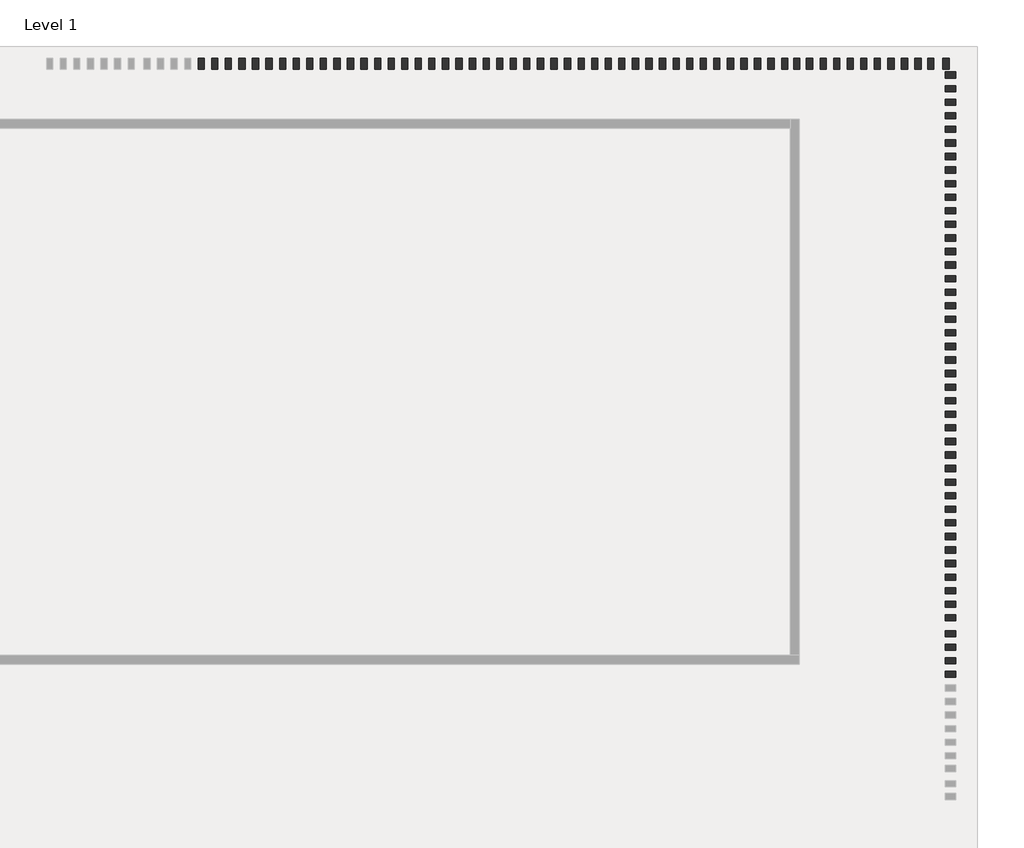
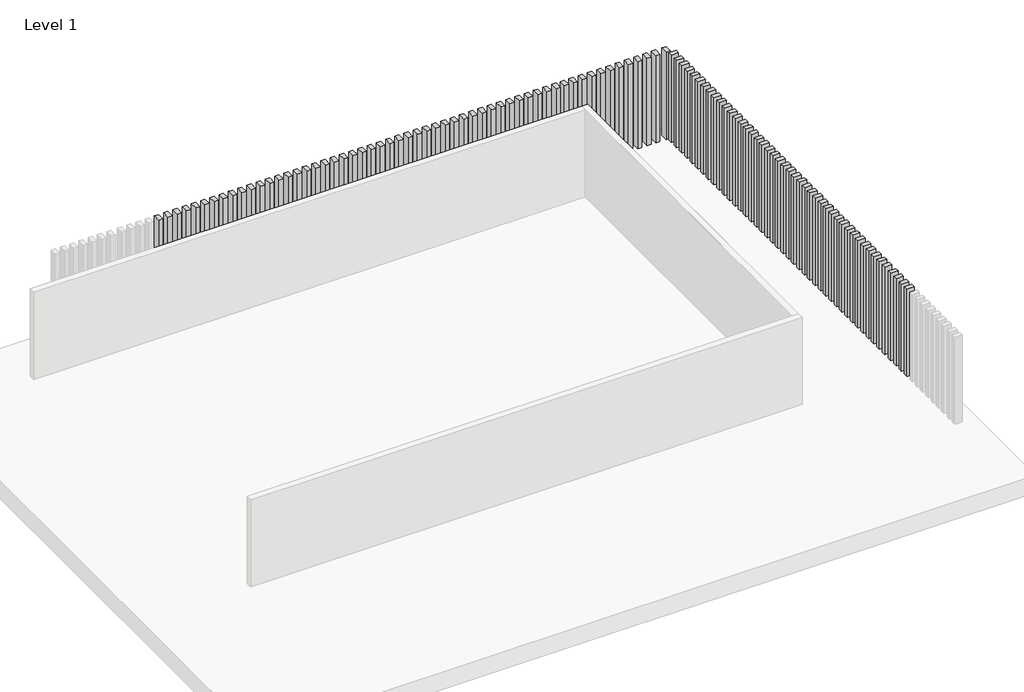
# One storey, part 3 of 3: 101 columns.
"""IFC4 building model written with IfcOpenShell, lengths in millimetres."""

from ifc_helpers import new_model, si_unit, origin, place, context, project, spatial, transform, mapped, element, save
from components import wood_timber_column_6_x_10_8585acab

model = new_model("IFC4")

# Units and contexts
model_context = context("Model", 3, world=origin())
ifc_project = project(units=[si_unit("LENGTHUNIT", "METRE", prefix="MILLI")], contexts=[model_context])

# Site, building, storey
site = spatial("IfcSite", under=ifc_project)
building = spatial("IfcBuilding", under=site)
storey = spatial("IfcBuildingStorey", under=building, Name="Level 1", Elevation=0.0)

# Columns
placement = place(None, origin())
wood_timber_column_6_x_10_shape = wood_timber_column_6_x_10_8585acab(model_context)
element("IfcColumn", 1, ObjectType="Wood Timber Column : 6 x 10", at=placement, inside=storey, context=model_context, shape_type="MappedRepresentation", body=[
    mapped(wood_timber_column_6_x_10_shape, transform((6080.1851725, 13462.6652966, 0.0), x_axis=(0.0, 1.0, 0.0), y_axis=(-1.0000000000000002, 0.0, 0.0), z_axis=(0.0, 0.0, 1.0000000000000002))),
])
element("IfcColumn", 2, ObjectType="Wood Timber Column : 6 x 10", at=placement, inside=storey, context=model_context, shape_type="MappedRepresentation", body=[
    mapped(wood_timber_column_6_x_10_shape, transform((6080.1851725, 13157.8652966, 0.0), x_axis=(0.0, 1.0, 0.0), y_axis=(-1.0000000000000002, 0.0, 0.0), z_axis=(0.0, 0.0, 1.0000000000000002))),
])
element("IfcColumn", 3, ObjectType="Wood Timber Column : 6 x 10", at=placement, inside=storey, context=model_context, shape_type="MappedRepresentation", body=[
    mapped(wood_timber_column_6_x_10_shape, transform((6080.1851725, 12853.0652966, 0.0), x_axis=(0.0, 1.0, 0.0), y_axis=(-1.0000000000000002, 0.0, 0.0), z_axis=(0.0, 0.0, 1.0000000000000002))),
])
element("IfcColumn", 4, ObjectType="Wood Timber Column : 6 x 10", at=placement, inside=storey, context=model_context, shape_type="MappedRepresentation", body=[
    mapped(wood_timber_column_6_x_10_shape, transform((6080.1851725, 12548.2652966, 0.0), x_axis=(0.0, 1.0, 0.0), y_axis=(-1.0000000000000002, 0.0, 0.0), z_axis=(0.0, 0.0, 1.0000000000000002))),
])
element("IfcColumn", 5, ObjectType="Wood Timber Column : 6 x 10", at=placement, inside=storey, context=model_context, shape_type="MappedRepresentation", body=[
    mapped(wood_timber_column_6_x_10_shape, transform((6080.1851725, 12243.4652966, 0.0), x_axis=(0.0, 1.0, 0.0), y_axis=(-1.0000000000000002, 0.0, 0.0), z_axis=(0.0, 0.0, 1.0000000000000002))),
])
element("IfcColumn", 6, ObjectType="Wood Timber Column : 6 x 10", at=placement, inside=storey, context=model_context, shape_type="MappedRepresentation", body=[
    mapped(wood_timber_column_6_x_10_shape, transform((6080.1851725, 11938.6652966, 0.0), x_axis=(0.0, 1.0, 0.0), y_axis=(-1.0000000000000002, 0.0, 0.0), z_axis=(0.0, 0.0, 1.0000000000000002))),
])
element("IfcColumn", 7, ObjectType="Wood Timber Column : 6 x 10", at=placement, inside=storey, context=model_context, shape_type="MappedRepresentation", body=[
    mapped(wood_timber_column_6_x_10_shape, transform((6080.1851725, 11633.8652966, 0.0), x_axis=(0.0, 1.0, 0.0), y_axis=(-1.0000000000000002, 0.0, 0.0), z_axis=(0.0, 0.0, 1.0000000000000002))),
])
element("IfcColumn", 8, ObjectType="Wood Timber Column : 6 x 10", at=placement, inside=storey, context=model_context, shape_type="MappedRepresentation", body=[
    mapped(wood_timber_column_6_x_10_shape, transform((6080.1851725, 11329.0652966, 0.0), x_axis=(0.0, 1.0, 0.0), y_axis=(-1.0000000000000002, 0.0, 0.0), z_axis=(0.0, 0.0, 1.0000000000000002))),
])
element("IfcColumn", 9, ObjectType="Wood Timber Column : 6 x 10", at=placement, inside=storey, context=model_context, shape_type="MappedRepresentation", body=[
    mapped(wood_timber_column_6_x_10_shape, transform((6080.1851725, 11024.2652966, 0.0), x_axis=(0.0, 1.0, 0.0), y_axis=(-1.0000000000000002, 0.0, 0.0), z_axis=(0.0, 0.0, 1.0000000000000002))),
])
element("IfcColumn", 10, ObjectType="Wood Timber Column : 6 x 10", at=placement, inside=storey, context=model_context, shape_type="MappedRepresentation", body=[
    mapped(wood_timber_column_6_x_10_shape, transform((6080.1851725, 10719.4652966, 0.0), x_axis=(0.0, 1.0, 0.0), y_axis=(-1.0000000000000002, 0.0, 0.0), z_axis=(0.0, 0.0, 1.0000000000000002))),
])
element("IfcColumn", 11, ObjectType="Wood Timber Column : 6 x 10", at=placement, inside=storey, context=model_context, shape_type="MappedRepresentation", body=[
    mapped(wood_timber_column_6_x_10_shape, transform((6080.1851725, 10414.6652966, 0.0), x_axis=(0.0, 1.0, 0.0), y_axis=(-1.0000000000000002, 0.0, 0.0), z_axis=(0.0, 0.0, 1.0000000000000002))),
])
element("IfcColumn", 12, ObjectType="Wood Timber Column : 6 x 10", at=placement, inside=storey, context=model_context, shape_type="MappedRepresentation", body=[
    mapped(wood_timber_column_6_x_10_shape, transform((6080.1851725, 10109.8652966, 0.0), x_axis=(0.0, 1.0, 0.0), y_axis=(-1.0000000000000002, 0.0, 0.0), z_axis=(0.0, 0.0, 1.0000000000000002))),
])
element("IfcColumn", 13, ObjectType="Wood Timber Column : 6 x 10", at=placement, inside=storey, context=model_context, shape_type="MappedRepresentation", body=[
    mapped(wood_timber_column_6_x_10_shape, transform((6080.1851725, 9805.0652966, 0.0), x_axis=(0.0, 1.0, 0.0), y_axis=(-1.0000000000000002, 0.0, 0.0), z_axis=(0.0, 0.0, 1.0000000000000002))),
])
element("IfcColumn", 14, ObjectType="Wood Timber Column : 6 x 10", at=placement, inside=storey, context=model_context, shape_type="MappedRepresentation", body=[
    mapped(wood_timber_column_6_x_10_shape, transform((6080.1851725, 9500.2652966, 0.0), x_axis=(0.0, 1.0, 0.0), y_axis=(-1.0000000000000002, 0.0, 0.0), z_axis=(0.0, 0.0, 1.0000000000000002))),
])
element("IfcColumn", 15, ObjectType="Wood Timber Column : 6 x 10", at=placement, inside=storey, context=model_context, shape_type="MappedRepresentation", body=[
    mapped(wood_timber_column_6_x_10_shape, transform((6080.1851725, 9195.4652966, 0.0), x_axis=(0.0, 1.0, 0.0), y_axis=(-1.0000000000000002, 0.0, 0.0), z_axis=(0.0, 0.0, 1.0000000000000002))),
])
element("IfcColumn", 16, ObjectType="Wood Timber Column : 6 x 10", at=placement, inside=storey, context=model_context, shape_type="MappedRepresentation", body=[
    mapped(wood_timber_column_6_x_10_shape, transform((6080.1851725, 8890.6652966, 0.0), x_axis=(0.0, 1.0, 0.0), y_axis=(-1.0000000000000002, 0.0, 0.0), z_axis=(0.0, 0.0, 1.0000000000000002))),
])
element("IfcColumn", 17, ObjectType="Wood Timber Column : 6 x 10", at=placement, inside=storey, context=model_context, shape_type="MappedRepresentation", body=[
    mapped(wood_timber_column_6_x_10_shape, transform((6080.1851725, 8585.8652966, 0.0), x_axis=(0.0, 1.0, 0.0), y_axis=(-1.0000000000000002, 0.0, 0.0), z_axis=(0.0, 0.0, 1.0000000000000002))),
])
element("IfcColumn", 18, ObjectType="Wood Timber Column : 6 x 10", at=placement, inside=storey, context=model_context, shape_type="MappedRepresentation", body=[
    mapped(wood_timber_column_6_x_10_shape, transform((6080.1851725, 8281.0652966, 0.0), x_axis=(0.0, 1.0, 0.0), y_axis=(-1.0000000000000002, 0.0, 0.0), z_axis=(0.0, 0.0, 1.0000000000000002))),
])
element("IfcColumn", 19, ObjectType="Wood Timber Column : 6 x 10", at=placement, inside=storey, context=model_context, shape_type="MappedRepresentation", body=[
    mapped(wood_timber_column_6_x_10_shape, transform((6080.1851725, 7976.2652966, 0.0), x_axis=(0.0, 1.0, 0.0), y_axis=(-1.0000000000000002, 0.0, 0.0), z_axis=(0.0, 0.0, 1.0000000000000002))),
])
element("IfcColumn", 20, ObjectType="Wood Timber Column : 6 x 10", at=placement, inside=storey, context=model_context, shape_type="MappedRepresentation", body=[
    mapped(wood_timber_column_6_x_10_shape, transform((6080.1851725, 7671.4652966, 0.0), x_axis=(0.0, 1.0, 0.0), y_axis=(-1.0000000000000002, 0.0, 0.0), z_axis=(0.0, 0.0, 1.0000000000000002))),
])
element("IfcColumn", 21, ObjectType="Wood Timber Column : 6 x 10", at=placement, inside=storey, context=model_context, shape_type="MappedRepresentation", body=[
    mapped(wood_timber_column_6_x_10_shape, transform((6080.1851725, 7366.6652966, 0.0), x_axis=(0.0, 1.0, 0.0), y_axis=(-1.0000000000000002, 0.0, 0.0), z_axis=(0.0, 0.0, 1.0000000000000002))),
])
element("IfcColumn", 22, ObjectType="Wood Timber Column : 6 x 10", at=placement, inside=storey, context=model_context, shape_type="MappedRepresentation", body=[
    mapped(wood_timber_column_6_x_10_shape, transform((6080.1851725, 7061.8652966, 0.0), x_axis=(0.0, 1.0, 0.0), y_axis=(-1.0000000000000002, 0.0, 0.0), z_axis=(0.0, 0.0, 1.0000000000000002))),
])
element("IfcColumn", 23, ObjectType="Wood Timber Column : 6 x 10", at=placement, inside=storey, context=model_context, shape_type="MappedRepresentation", body=[
    mapped(wood_timber_column_6_x_10_shape, transform((6080.1851725, 6757.0652966, 0.0), x_axis=(0.0, 1.0, 0.0), y_axis=(-1.0000000000000002, 0.0, 0.0), z_axis=(0.0, 0.0, 1.0000000000000002))),
])
element("IfcColumn", 24, ObjectType="Wood Timber Column : 6 x 10", at=placement, inside=storey, context=model_context, shape_type="MappedRepresentation", body=[
    mapped(wood_timber_column_6_x_10_shape, transform((6080.1851725, 6452.2652966, 0.0), x_axis=(0.0, 1.0, 0.0), y_axis=(-1.0000000000000002, 0.0, 0.0), z_axis=(0.0, 0.0, 1.0000000000000002))),
])
element("IfcColumn", 25, ObjectType="Wood Timber Column : 6 x 10", at=placement, inside=storey, context=model_context, shape_type="MappedRepresentation", body=[
    mapped(wood_timber_column_6_x_10_shape, transform((6080.1851725, 6147.4652966, 0.0), x_axis=(0.0, 1.0, 0.0), y_axis=(-1.0000000000000002, 0.0, 0.0), z_axis=(0.0, 0.0, 1.0000000000000002))),
])
element("IfcColumn", 26, ObjectType="Wood Timber Column : 6 x 10", at=placement, inside=storey, context=model_context, shape_type="MappedRepresentation", body=[
    mapped(wood_timber_column_6_x_10_shape, transform((6080.1851725, 5842.6652966, 0.0), x_axis=(0.0, 1.0, 0.0), y_axis=(-1.0000000000000002, 0.0, 0.0), z_axis=(0.0, 0.0, 1.0000000000000002))),
])
element("IfcColumn", 27, ObjectType="Wood Timber Column : 6 x 10", at=placement, inside=storey, context=model_context, shape_type="MappedRepresentation", body=[
    mapped(wood_timber_column_6_x_10_shape, transform((6080.1851725, 5537.8652966, 0.0), x_axis=(0.0, 1.0, 0.0), y_axis=(-1.0000000000000002, 0.0, 0.0), z_axis=(0.0, 0.0, 1.0000000000000002))),
])
element("IfcColumn", 28, ObjectType="Wood Timber Column : 6 x 10", at=placement, inside=storey, context=model_context, shape_type="MappedRepresentation", body=[
    mapped(wood_timber_column_6_x_10_shape, transform((6080.1851725, 5233.0652966, 0.0), x_axis=(0.0, 1.0, 0.0), y_axis=(-1.0000000000000002, 0.0, 0.0), z_axis=(0.0, 0.0, 1.0000000000000002))),
])
element("IfcColumn", 29, ObjectType="Wood Timber Column : 6 x 10", at=placement, inside=storey, context=model_context, shape_type="MappedRepresentation", body=[
    mapped(wood_timber_column_6_x_10_shape, transform((6080.1851725, 4928.2652966, 0.0), x_axis=(0.0, 1.0, 0.0), y_axis=(-1.0000000000000002, 0.0, 0.0), z_axis=(0.0, 0.0, 1.0000000000000002))),
])
element("IfcColumn", 30, ObjectType="Wood Timber Column : 6 x 10", at=placement, inside=storey, context=model_context, shape_type="MappedRepresentation", body=[
    mapped(wood_timber_column_6_x_10_shape, transform((6080.1851725, 4623.4652966, 0.0), x_axis=(0.0, 1.0, 0.0), y_axis=(-1.0000000000000002, 0.0, 0.0), z_axis=(0.0, 0.0, 1.0000000000000002))),
])
element("IfcColumn", 31, ObjectType="Wood Timber Column : 6 x 10", at=placement, inside=storey, context=model_context, shape_type="MappedRepresentation", body=[
    mapped(wood_timber_column_6_x_10_shape, transform((6080.1851725, 4318.6652966, 0.0), x_axis=(0.0, 1.0, 0.0), y_axis=(-1.0000000000000002, 0.0, 0.0), z_axis=(0.0, 0.0, 1.0000000000000002))),
])
element("IfcColumn", 32, ObjectType="Wood Timber Column : 6 x 10", at=placement, inside=storey, context=model_context, shape_type="MappedRepresentation", body=[
    mapped(wood_timber_column_6_x_10_shape, transform((6080.1851725, 4013.8652966, 0.0), x_axis=(0.0, 1.0, 0.0), y_axis=(-1.0000000000000002, 0.0, 0.0), z_axis=(0.0, 0.0, 1.0000000000000002))),
])
element("IfcColumn", 33, ObjectType="Wood Timber Column : 6 x 10", at=placement, inside=storey, context=model_context, shape_type="MappedRepresentation", body=[
    mapped(wood_timber_column_6_x_10_shape, transform((6080.1851725, 3709.0652966, 0.0), x_axis=(0.0, 1.0, 0.0), y_axis=(-1.0000000000000002, 0.0, 0.0), z_axis=(0.0, 0.0, 1.0000000000000002))),
])
element("IfcColumn", 34, ObjectType="Wood Timber Column : 6 x 10", at=placement, inside=storey, context=model_context, shape_type="MappedRepresentation", body=[
    mapped(wood_timber_column_6_x_10_shape, transform((6080.1851725, 3404.2652966, 0.0), x_axis=(0.0, 1.0, 0.0), y_axis=(-1.0000000000000002, 0.0, 0.0), z_axis=(0.0, 0.0, 1.0000000000000002))),
])
element("IfcColumn", 35, ObjectType="Wood Timber Column : 6 x 10", at=placement, inside=storey, context=model_context, shape_type="MappedRepresentation", body=[
    mapped(wood_timber_column_6_x_10_shape, transform((6080.1851725, 3099.4652966, 0.0), x_axis=(0.0, 1.0, 0.0), y_axis=(-1.0000000000000002, 0.0, 0.0), z_axis=(0.0, 0.0, 1.0000000000000002))),
])
element("IfcColumn", 36, ObjectType="Wood Timber Column : 6 x 10", at=placement, inside=storey, context=model_context, shape_type="MappedRepresentation", body=[
    mapped(wood_timber_column_6_x_10_shape, transform((6080.1851725, 2794.6652966, 0.0), x_axis=(0.0, 1.0, 0.0), y_axis=(-1.0000000000000002, 0.0, 0.0), z_axis=(0.0, 0.0, 1.0000000000000002))),
])
element("IfcColumn", 37, ObjectType="Wood Timber Column : 6 x 10", at=placement, inside=storey, context=model_context, shape_type="MappedRepresentation", body=[
    mapped(wood_timber_column_6_x_10_shape, transform((6080.1851725, 2489.8652966, 0.0), x_axis=(0.0, 1.0, 0.0), y_axis=(-1.0000000000000002, 0.0, 0.0), z_axis=(0.0, 0.0, 1.0000000000000002))),
])
element("IfcColumn", 38, ObjectType="Wood Timber Column : 6 x 10", at=placement, inside=storey, context=model_context, shape_type="MappedRepresentation", body=[
    mapped(wood_timber_column_6_x_10_shape, transform((6080.1851725, 2185.0652966, 0.0), x_axis=(0.0, 1.0, 0.0), y_axis=(-1.0000000000000002, 0.0, 0.0), z_axis=(0.0, 0.0, 1.0000000000000002))),
])
element("IfcColumn", 39, ObjectType="Wood Timber Column : 6 x 10", at=placement, inside=storey, context=model_context, shape_type="MappedRepresentation", body=[
    mapped(wood_timber_column_6_x_10_shape, transform((6080.1851725, 1880.2652966, 0.0), x_axis=(0.0, 1.0, 0.0), y_axis=(-1.0000000000000002, 0.0, 0.0), z_axis=(0.0, 0.0, 1.0000000000000002))),
])
element("IfcColumn", 40, ObjectType="Wood Timber Column : 6 x 10", at=placement, inside=storey, context=model_context, shape_type="MappedRepresentation", body=[
    mapped(wood_timber_column_6_x_10_shape, transform((6080.1851725, 1575.4652966, 0.0), x_axis=(0.0, 1.0, 0.0), y_axis=(-1.0000000000000002, 0.0, 0.0), z_axis=(0.0, 0.0, 1.0000000000000002))),
])
element("IfcColumn", 41, ObjectType="Wood Timber Column : 6 x 10", at=placement, inside=storey, context=model_context, shape_type="MappedRepresentation", body=[
    mapped(wood_timber_column_6_x_10_shape, transform((6080.1851725, 1270.6652966, 0.0), x_axis=(0.0, 1.0, 0.0), y_axis=(-1.0000000000000002, 0.0, 0.0), z_axis=(0.0, 0.0, 1.0000000000000002))),
])
element("IfcColumn", 42, ObjectType="Wood Timber Column : 6 x 10", at=placement, inside=storey, context=model_context, shape_type="MappedRepresentation", body=[
    mapped(wood_timber_column_6_x_10_shape, transform((6080.1851725, 915.0652966, 0.0), x_axis=(0.0, 1.0, 0.0), y_axis=(-1.0000000000000002, 0.0, 0.0), z_axis=(0.0, 0.0, 1.0000000000000002))),
])
element("IfcColumn", 43, ObjectType="Wood Timber Column : 6 x 10", at=placement, inside=storey, context=model_context, shape_type="MappedRepresentation", body=[
    mapped(wood_timber_column_6_x_10_shape, transform((6080.1851725, 610.2652966, 0.0), x_axis=(0.0, 1.0, 0.0), y_axis=(-1.0000000000000002, 0.0, 0.0), z_axis=(0.0, 0.0, 1.0000000000000002))),
])
element("IfcColumn", 44, ObjectType="Wood Timber Column : 6 x 10", at=placement, inside=storey, context=model_context, shape_type="MappedRepresentation", body=[
    mapped(wood_timber_column_6_x_10_shape, transform((6080.1851725, 305.4652966, 0.0), x_axis=(0.0, 1.0, 0.0), y_axis=(-1.0000000000000002, 0.0, 0.0), z_axis=(0.0, 0.0, 1.0000000000000002))),
])
element("IfcColumn", 45, ObjectType="Wood Timber Column : 6 x 10", at=placement, inside=storey, context=model_context, shape_type="MappedRepresentation", body=[
    mapped(wood_timber_column_6_x_10_shape, transform((6080.1851725, 0.6652966, 0.0), x_axis=(0.0, 1.0, 0.0), y_axis=(-1.0000000000000002, 0.0, 0.0), z_axis=(0.0, 0.0, 1.0000000000000002))),
])
element("IfcColumn", 46, ObjectType="Wood Timber Column : 6 x 10", at=placement, inside=storey, context=model_context, shape_type="MappedRepresentation", body=[
    mapped(wood_timber_column_6_x_10_shape, transform((2625.7851725, 13716.6652966, 0.0), x_axis=(1.0, 0.0, 0.0), y_axis=(0.0, 1.0, 0.0), z_axis=(0.0, 0.0, 1.0))),
])
element("IfcColumn", 47, ObjectType="Wood Timber Column : 6 x 10", at=placement, inside=storey, context=model_context, shape_type="MappedRepresentation", body=[
    mapped(wood_timber_column_6_x_10_shape, transform((2352.7351725, 13716.6652966, 0.0), x_axis=(1.0, 0.0, 0.0), y_axis=(0.0, 1.0, 0.0), z_axis=(0.0, 0.0, 1.0))),
])
element("IfcColumn", 48, ObjectType="Wood Timber Column : 6 x 10", at=placement, inside=storey, context=model_context, shape_type="MappedRepresentation", body=[
    mapped(wood_timber_column_6_x_10_shape, transform((2047.9351725, 13716.6652966, 0.0), x_axis=(1.0, 0.0, 0.0), y_axis=(0.0, 1.0, 0.0), z_axis=(0.0, 0.0, 1.0))),
])
element("IfcColumn", 49, ObjectType="Wood Timber Column : 6 x 10", at=placement, inside=storey, context=model_context, shape_type="MappedRepresentation", body=[
    mapped(wood_timber_column_6_x_10_shape, transform((1743.1351725, 13716.6652966, 0.0), x_axis=(1.0, 0.0, 0.0), y_axis=(0.0, 1.0, 0.0), z_axis=(0.0, 0.0, 1.0))),
])
element("IfcColumn", 50, ObjectType="Wood Timber Column : 6 x 10", at=placement, inside=storey, context=model_context, shape_type="MappedRepresentation", body=[
    mapped(wood_timber_column_6_x_10_shape, transform((1438.3351725, 13716.6652966, 0.0), x_axis=(1.0, 0.0, 0.0), y_axis=(0.0, 1.0, 0.0), z_axis=(0.0, 0.0, 1.0))),
])
element("IfcColumn", 51, ObjectType="Wood Timber Column : 6 x 10", at=placement, inside=storey, context=model_context, shape_type="MappedRepresentation", body=[
    mapped(wood_timber_column_6_x_10_shape, transform((1133.5351725, 13716.6652966, 0.0), x_axis=(1.0, 0.0, 0.0), y_axis=(0.0, 1.0, 0.0), z_axis=(0.0, 0.0, 1.0))),
])
element("IfcColumn", 52, ObjectType="Wood Timber Column : 6 x 10", at=placement, inside=storey, context=model_context, shape_type="MappedRepresentation", body=[
    mapped(wood_timber_column_6_x_10_shape, transform((828.7351725, 13716.6652966, 0.0), x_axis=(1.0, 0.0, 0.0), y_axis=(0.0, 1.0, 0.0), z_axis=(0.0, 0.0, 1.0))),
])
element("IfcColumn", 53, ObjectType="Wood Timber Column : 6 x 10", at=placement, inside=storey, context=model_context, shape_type="MappedRepresentation", body=[
    mapped(wood_timber_column_6_x_10_shape, transform((523.9351725, 13716.6652966, 0.0), x_axis=(1.0, 0.0, 0.0), y_axis=(0.0, 1.0, 0.0), z_axis=(0.0, 0.0, 1.0))),
])
element("IfcColumn", 54, ObjectType="Wood Timber Column : 6 x 10", at=placement, inside=storey, context=model_context, shape_type="MappedRepresentation", body=[
    mapped(wood_timber_column_6_x_10_shape, transform((219.1351725, 13716.6652966, 0.0), x_axis=(1.0, 0.0, 0.0), y_axis=(0.0, 1.0, 0.0), z_axis=(0.0, 0.0, 1.0))),
])
element("IfcColumn", 55, ObjectType="Wood Timber Column : 6 x 10", at=placement, inside=storey, context=model_context, shape_type="MappedRepresentation", body=[
    mapped(wood_timber_column_6_x_10_shape, transform((-85.6648275, 13716.6652966, 0.0), x_axis=(1.0, 0.0, 0.0), y_axis=(0.0, 1.0, 0.0), z_axis=(0.0, 0.0, 1.0))),
])
element("IfcColumn", 56, ObjectType="Wood Timber Column : 6 x 10", at=placement, inside=storey, context=model_context, shape_type="MappedRepresentation", body=[
    mapped(wood_timber_column_6_x_10_shape, transform((-390.4648275, 13716.6652966, 0.0), x_axis=(1.0, 0.0, 0.0), y_axis=(0.0, 1.0, 0.0), z_axis=(0.0, 0.0, 1.0))),
])
element("IfcColumn", 57, ObjectType="Wood Timber Column : 6 x 10", at=placement, inside=storey, context=model_context, shape_type="MappedRepresentation", body=[
    mapped(wood_timber_column_6_x_10_shape, transform((-695.2648275, 13716.6652966, 0.0), x_axis=(1.0, 0.0, 0.0), y_axis=(0.0, 1.0, 0.0), z_axis=(0.0, 0.0, 1.0))),
])
element("IfcColumn", 58, ObjectType="Wood Timber Column : 6 x 10", at=placement, inside=storey, context=model_context, shape_type="MappedRepresentation", body=[
    mapped(wood_timber_column_6_x_10_shape, transform((-1000.0648275, 13716.6652966, 0.0), x_axis=(1.0, 0.0, 0.0), y_axis=(0.0, 1.0, 0.0), z_axis=(0.0, 0.0, 1.0))),
])
element("IfcColumn", 59, ObjectType="Wood Timber Column : 6 x 10", at=placement, inside=storey, context=model_context, shape_type="MappedRepresentation", body=[
    mapped(wood_timber_column_6_x_10_shape, transform((-1304.8648275, 13716.6652966, 0.0), x_axis=(1.0, 0.0, 0.0), y_axis=(0.0, 1.0, 0.0), z_axis=(0.0, 0.0, 1.0))),
])
element("IfcColumn", 60, ObjectType="Wood Timber Column : 6 x 10", at=placement, inside=storey, context=model_context, shape_type="MappedRepresentation", body=[
    mapped(wood_timber_column_6_x_10_shape, transform((-1609.6648275, 13716.6652966, 0.0), x_axis=(1.0, 0.0, 0.0), y_axis=(0.0, 1.0, 0.0), z_axis=(0.0, 0.0, 1.0))),
])
element("IfcColumn", 61, ObjectType="Wood Timber Column : 6 x 10", at=placement, inside=storey, context=model_context, shape_type="MappedRepresentation", body=[
    mapped(wood_timber_column_6_x_10_shape, transform((-1914.4648275, 13716.6652966, 0.0), x_axis=(1.0, 0.0, 0.0), y_axis=(0.0, 1.0, 0.0), z_axis=(0.0, 0.0, 1.0))),
])
element("IfcColumn", 62, ObjectType="Wood Timber Column : 6 x 10", at=placement, inside=storey, context=model_context, shape_type="MappedRepresentation", body=[
    mapped(wood_timber_column_6_x_10_shape, transform((-2219.2648275, 13716.6652966, 0.0), x_axis=(1.0, 0.0, 0.0), y_axis=(0.0, 1.0, 0.0), z_axis=(0.0, 0.0, 1.0))),
])
element("IfcColumn", 63, ObjectType="Wood Timber Column : 6 x 10", at=placement, inside=storey, context=model_context, shape_type="MappedRepresentation", body=[
    mapped(wood_timber_column_6_x_10_shape, transform((-2524.0648275, 13716.6652966, 0.0), x_axis=(1.0, 0.0, 0.0), y_axis=(0.0, 1.0, 0.0), z_axis=(0.0, 0.0, 1.0))),
])
element("IfcColumn", 64, ObjectType="Wood Timber Column : 6 x 10", at=placement, inside=storey, context=model_context, shape_type="MappedRepresentation", body=[
    mapped(wood_timber_column_6_x_10_shape, transform((-2828.8648275, 13716.6652966, 0.0), x_axis=(1.0, 0.0, 0.0), y_axis=(0.0, 1.0, 0.0), z_axis=(0.0, 0.0, 1.0))),
])
element("IfcColumn", 65, ObjectType="Wood Timber Column : 6 x 10", at=placement, inside=storey, context=model_context, shape_type="MappedRepresentation", body=[
    mapped(wood_timber_column_6_x_10_shape, transform((-3133.6648275, 13716.6652966, 0.0), x_axis=(1.0, 0.0, 0.0), y_axis=(0.0, 1.0, 0.0), z_axis=(0.0, 0.0, 1.0))),
])
element("IfcColumn", 66, ObjectType="Wood Timber Column : 6 x 10", at=placement, inside=storey, context=model_context, shape_type="MappedRepresentation", body=[
    mapped(wood_timber_column_6_x_10_shape, transform((-3438.4648275, 13716.6652966, 0.0), x_axis=(1.0, 0.0, 0.0), y_axis=(0.0, 1.0, 0.0), z_axis=(0.0, 0.0, 1.0))),
])
element("IfcColumn", 67, ObjectType="Wood Timber Column : 6 x 10", at=placement, inside=storey, context=model_context, shape_type="MappedRepresentation", body=[
    mapped(wood_timber_column_6_x_10_shape, transform((-3743.2648275, 13716.6652966, 0.0), x_axis=(1.0, 0.0, 0.0), y_axis=(0.0, 1.0, 0.0), z_axis=(0.0, 0.0, 1.0))),
])
element("IfcColumn", 68, ObjectType="Wood Timber Column : 6 x 10", at=placement, inside=storey, context=model_context, shape_type="MappedRepresentation", body=[
    mapped(wood_timber_column_6_x_10_shape, transform((-4048.0648275, 13716.6652966, 0.0), x_axis=(1.0, 0.0, 0.0), y_axis=(0.0, 1.0, 0.0), z_axis=(0.0, 0.0, 1.0))),
])
element("IfcColumn", 69, ObjectType="Wood Timber Column : 6 x 10", at=placement, inside=storey, context=model_context, shape_type="MappedRepresentation", body=[
    mapped(wood_timber_column_6_x_10_shape, transform((-4352.8648275, 13716.6652966, 0.0), x_axis=(1.0, 0.0, 0.0), y_axis=(0.0, 1.0, 0.0), z_axis=(0.0, 0.0, 1.0))),
])
element("IfcColumn", 70, ObjectType="Wood Timber Column : 6 x 10", at=placement, inside=storey, context=model_context, shape_type="MappedRepresentation", body=[
    mapped(wood_timber_column_6_x_10_shape, transform((-4657.6648275, 13716.6652966, 0.0), x_axis=(1.0, 0.0, 0.0), y_axis=(0.0, 1.0, 0.0), z_axis=(0.0, 0.0, 1.0))),
])
element("IfcColumn", 71, ObjectType="Wood Timber Column : 6 x 10", at=placement, inside=storey, context=model_context, shape_type="MappedRepresentation", body=[
    mapped(wood_timber_column_6_x_10_shape, transform((-4962.4648275, 13716.6652966, 0.0), x_axis=(1.0, 0.0, 0.0), y_axis=(0.0, 1.0, 0.0), z_axis=(0.0, 0.0, 1.0))),
])
element("IfcColumn", 72, ObjectType="Wood Timber Column : 6 x 10", at=placement, inside=storey, context=model_context, shape_type="MappedRepresentation", body=[
    mapped(wood_timber_column_6_x_10_shape, transform((-5267.2648275, 13716.6652966, 0.0), x_axis=(1.0, 0.0, 0.0), y_axis=(0.0, 1.0, 0.0), z_axis=(0.0, 0.0, 1.0))),
])
element("IfcColumn", 73, ObjectType="Wood Timber Column : 6 x 10", at=placement, inside=storey, context=model_context, shape_type="MappedRepresentation", body=[
    mapped(wood_timber_column_6_x_10_shape, transform((-5572.0648275, 13716.6652966, 0.0), x_axis=(1.0, 0.0, 0.0), y_axis=(0.0, 1.0, 0.0), z_axis=(0.0, 0.0, 1.0))),
])
element("IfcColumn", 74, ObjectType="Wood Timber Column : 6 x 10", at=placement, inside=storey, context=model_context, shape_type="MappedRepresentation", body=[
    mapped(wood_timber_column_6_x_10_shape, transform((-5876.8648275, 13716.6652966, 0.0), x_axis=(1.0, 0.0, 0.0), y_axis=(0.0, 1.0, 0.0), z_axis=(0.0, 0.0, 1.0))),
])
element("IfcColumn", 75, ObjectType="Wood Timber Column : 6 x 10", at=placement, inside=storey, context=model_context, shape_type="MappedRepresentation", body=[
    mapped(wood_timber_column_6_x_10_shape, transform((-6181.6648275, 13716.6652966, 0.0), x_axis=(1.0, 0.0, 0.0), y_axis=(0.0, 1.0, 0.0), z_axis=(0.0, 0.0, 1.0))),
])
element("IfcColumn", 76, ObjectType="Wood Timber Column : 6 x 10", at=placement, inside=storey, context=model_context, shape_type="MappedRepresentation", body=[
    mapped(wood_timber_column_6_x_10_shape, transform((-6486.4648275, 13716.6652966, 0.0), x_axis=(1.0, 0.0, 0.0), y_axis=(0.0, 1.0, 0.0), z_axis=(0.0, 0.0, 1.0))),
])
element("IfcColumn", 77, ObjectType="Wood Timber Column : 6 x 10", at=placement, inside=storey, context=model_context, shape_type="MappedRepresentation", body=[
    mapped(wood_timber_column_6_x_10_shape, transform((-6791.2648275, 13716.6652966, 0.0), x_axis=(1.0, 0.0, 0.0), y_axis=(0.0, 1.0, 0.0), z_axis=(0.0, 0.0, 1.0))),
])
element("IfcColumn", 78, ObjectType="Wood Timber Column : 6 x 10", at=placement, inside=storey, context=model_context, shape_type="MappedRepresentation", body=[
    mapped(wood_timber_column_6_x_10_shape, transform((-7096.0648275, 13716.6652966, 0.0), x_axis=(1.0, 0.0, 0.0), y_axis=(0.0, 1.0, 0.0), z_axis=(0.0, 0.0, 1.0))),
])
element("IfcColumn", 79, ObjectType="Wood Timber Column : 6 x 10", at=placement, inside=storey, context=model_context, shape_type="MappedRepresentation", body=[
    mapped(wood_timber_column_6_x_10_shape, transform((-7400.8648275, 13716.6652966, 0.0), x_axis=(1.0, 0.0, 0.0), y_axis=(0.0, 1.0, 0.0), z_axis=(0.0, 0.0, 1.0))),
])
element("IfcColumn", 80, ObjectType="Wood Timber Column : 6 x 10", at=placement, inside=storey, context=model_context, shape_type="MappedRepresentation", body=[
    mapped(wood_timber_column_6_x_10_shape, transform((-7705.6648275, 13716.6652966, 0.0), x_axis=(1.0, 0.0, 0.0), y_axis=(0.0, 1.0, 0.0), z_axis=(0.0, 0.0, 1.0))),
])
element("IfcColumn", 81, ObjectType="Wood Timber Column : 6 x 10", at=placement, inside=storey, context=model_context, shape_type="MappedRepresentation", body=[
    mapped(wood_timber_column_6_x_10_shape, transform((-8010.4648275, 13716.6652966, 0.0), x_axis=(1.0, 0.0, 0.0), y_axis=(0.0, 1.0, 0.0), z_axis=(0.0, 0.0, 1.0))),
])
element("IfcColumn", 82, ObjectType="Wood Timber Column : 6 x 10", at=placement, inside=storey, context=model_context, shape_type="MappedRepresentation", body=[
    mapped(wood_timber_column_6_x_10_shape, transform((-8315.2648275, 13716.6652966, 0.0), x_axis=(1.0, 0.0, 0.0), y_axis=(0.0, 1.0, 0.0), z_axis=(0.0, 0.0, 1.0))),
])
element("IfcColumn", 83, ObjectType="Wood Timber Column : 6 x 10", at=placement, inside=storey, context=model_context, shape_type="MappedRepresentation", body=[
    mapped(wood_timber_column_6_x_10_shape, transform((-8620.0648275, 13716.6652966, 0.0), x_axis=(1.0, 0.0, 0.0), y_axis=(0.0, 1.0, 0.0), z_axis=(0.0, 0.0, 1.0))),
])
element("IfcColumn", 84, ObjectType="Wood Timber Column : 6 x 10", at=placement, inside=storey, context=model_context, shape_type="MappedRepresentation", body=[
    mapped(wood_timber_column_6_x_10_shape, transform((-8924.8648275, 13716.6652966, 0.0), x_axis=(1.0, 0.0, 0.0), y_axis=(0.0, 1.0, 0.0), z_axis=(0.0, 0.0, 1.0))),
])
element("IfcColumn", 85, ObjectType="Wood Timber Column : 6 x 10", at=placement, inside=storey, context=model_context, shape_type="MappedRepresentation", body=[
    mapped(wood_timber_column_6_x_10_shape, transform((-9229.6648275, 13716.6652966, 0.0), x_axis=(1.0, 0.0, 0.0), y_axis=(0.0, 1.0, 0.0), z_axis=(0.0, 0.0, 1.0))),
])
element("IfcColumn", 86, ObjectType="Wood Timber Column : 6 x 10", at=placement, inside=storey, context=model_context, shape_type="MappedRepresentation", body=[
    mapped(wood_timber_column_6_x_10_shape, transform((-9534.4648275, 13716.6652966, 0.0), x_axis=(1.0, 0.0, 0.0), y_axis=(0.0, 1.0, 0.0), z_axis=(0.0, 0.0, 1.0))),
])
element("IfcColumn", 87, ObjectType="Wood Timber Column : 6 x 10", at=placement, inside=storey, context=model_context, shape_type="MappedRepresentation", body=[
    mapped(wood_timber_column_6_x_10_shape, transform((-9839.2648275, 13716.6652966, 0.0), x_axis=(1.0, 0.0, 0.0), y_axis=(0.0, 1.0, 0.0), z_axis=(0.0, 0.0, 1.0))),
])
element("IfcColumn", 88, ObjectType="Wood Timber Column : 6 x 10", at=placement, inside=storey, context=model_context, shape_type="MappedRepresentation", body=[
    mapped(wood_timber_column_6_x_10_shape, transform((-10144.0648275, 13716.6652966, 0.0), x_axis=(1.0, 0.0, 0.0), y_axis=(0.0, 1.0, 0.0), z_axis=(0.0, 0.0, 1.0))),
])
element("IfcColumn", 89, ObjectType="Wood Timber Column : 6 x 10", at=placement, inside=storey, context=model_context, shape_type="MappedRepresentation", body=[
    mapped(wood_timber_column_6_x_10_shape, transform((-10448.8648275, 13716.6652966, 0.0), x_axis=(1.0, 0.0, 0.0), y_axis=(0.0, 1.0, 0.0), z_axis=(0.0, 0.0, 1.0))),
])
element("IfcColumn", 90, ObjectType="Wood Timber Column : 6 x 10", at=placement, inside=storey, context=model_context, shape_type="MappedRepresentation", body=[
    mapped(wood_timber_column_6_x_10_shape, transform((-10753.6648275, 13716.6652966, 0.0), x_axis=(1.0, 0.0, 0.0), y_axis=(0.0, 1.0, 0.0), z_axis=(0.0, 0.0, 1.0))),
])
element("IfcColumn", 91, ObjectType="Wood Timber Column : 6 x 10", at=placement, inside=storey, context=model_context, shape_type="MappedRepresentation", body=[
    mapped(wood_timber_column_6_x_10_shape, transform((5978.5851725, 13716.6652966, 0.0), x_axis=(1.0, 0.0, 0.0), y_axis=(0.0, 1.0, 0.0), z_axis=(0.0, 0.0, 1.0))),
])
element("IfcColumn", 92, ObjectType="Wood Timber Column : 6 x 10", at=placement, inside=storey, context=model_context, shape_type="MappedRepresentation", body=[
    mapped(wood_timber_column_6_x_10_shape, transform((5635.6851725, 13716.6652966, 0.0), x_axis=(1.0, 0.0, 0.0), y_axis=(0.0, 1.0, 0.0), z_axis=(0.0, 0.0, 1.0))),
])
element("IfcColumn", 93, ObjectType="Wood Timber Column : 6 x 10", at=placement, inside=storey, context=model_context, shape_type="MappedRepresentation", body=[
    mapped(wood_timber_column_6_x_10_shape, transform((5349.9351725, 13716.6652966, 0.0), x_axis=(1.0, 0.0, 0.0), y_axis=(0.0, 1.0, 0.0), z_axis=(0.0, 0.0, 1.0))),
])
element("IfcColumn", 94, ObjectType="Wood Timber Column : 6 x 10", at=placement, inside=storey, context=model_context, shape_type="MappedRepresentation", body=[
    mapped(wood_timber_column_6_x_10_shape, transform((5045.1351725, 13716.6652966, 0.0), x_axis=(1.0, 0.0, 0.0), y_axis=(0.0, 1.0, 0.0), z_axis=(0.0, 0.0, 1.0))),
])
element("IfcColumn", 95, ObjectType="Wood Timber Column : 6 x 10", at=placement, inside=storey, context=model_context, shape_type="MappedRepresentation", body=[
    mapped(wood_timber_column_6_x_10_shape, transform((4740.3351725, 13716.6652966, 0.0), x_axis=(1.0, 0.0, 0.0), y_axis=(0.0, 1.0, 0.0), z_axis=(0.0, 0.0, 1.0))),
])
element("IfcColumn", 96, ObjectType="Wood Timber Column : 6 x 10", at=placement, inside=storey, context=model_context, shape_type="MappedRepresentation", body=[
    mapped(wood_timber_column_6_x_10_shape, transform((4435.5351725, 13716.6652966, 0.0), x_axis=(1.0, 0.0, 0.0), y_axis=(0.0, 1.0, 0.0), z_axis=(0.0, 0.0, 1.0))),
])
element("IfcColumn", 97, ObjectType="Wood Timber Column : 6 x 10", at=placement, inside=storey, context=model_context, shape_type="MappedRepresentation", body=[
    mapped(wood_timber_column_6_x_10_shape, transform((4130.7351725, 13716.6652966, 0.0), x_axis=(1.0, 0.0, 0.0), y_axis=(0.0, 1.0, 0.0), z_axis=(0.0, 0.0, 1.0))),
])
element("IfcColumn", 98, ObjectType="Wood Timber Column : 6 x 10", at=placement, inside=storey, context=model_context, shape_type="MappedRepresentation", body=[
    mapped(wood_timber_column_6_x_10_shape, transform((3825.9351725, 13716.6652966, 0.0), x_axis=(1.0, 0.0, 0.0), y_axis=(0.0, 1.0, 0.0), z_axis=(0.0, 0.0, 1.0))),
])
element("IfcColumn", 99, ObjectType="Wood Timber Column : 6 x 10", at=placement, inside=storey, context=model_context, shape_type="MappedRepresentation", body=[
    mapped(wood_timber_column_6_x_10_shape, transform((3521.1351725, 13716.6652966, 0.0), x_axis=(1.0, 0.0, 0.0), y_axis=(0.0, 1.0, 0.0), z_axis=(0.0, 0.0, 1.0))),
])
element("IfcColumn", 100, ObjectType="Wood Timber Column : 6 x 10", at=placement, inside=storey, context=model_context, shape_type="MappedRepresentation", body=[
    mapped(wood_timber_column_6_x_10_shape, transform((3216.3351725, 13716.6652966, 0.0), x_axis=(1.0, 0.0, 0.0), y_axis=(0.0, 1.0, 0.0), z_axis=(0.0, 0.0, 1.0))),
])
element("IfcColumn", 101, ObjectType="Wood Timber Column : 6 x 10", at=placement, inside=storey, context=model_context, shape_type="MappedRepresentation", body=[
    mapped(wood_timber_column_6_x_10_shape, transform((2911.5351725, 13716.6652966, 0.0), x_axis=(1.0, 0.0, 0.0), y_axis=(0.0, 1.0, 0.0), z_axis=(0.0, 0.0, 1.0))),
])

save(model, "model.ifc")

# Revit data of these elements
# Type "Wood Timber Column : 6 x 10"
#   Assembly Code = "B1010200"
#   Depth = 0' - 9 1/2"
#   Width = 0' - 5 1/2"
#   Material = Softwood, Lumber
# Elements 1, 2, 3, 4, 5, 6, 7, 8, 9, 10, 11, 12, 13, 14, 15, 16, 17, 18, 19, 20, 21, 22, 23, 24, 25, 26, 27, 28, 29, 30, 31, 32, 33, 34, 35, 36, 37, 38, 39, 40, 41, 42, 43, 44, 45, 46, 47, 48, 49, 50, 51, 52, 53, 54, 55, 56, 57, 58, 59, 60, 61, 62, 63, 64, 65, 66, 67, 68, 69, 70, 71, 72, 73, 74, 75, 76, 77, 78, 79, 80, 81, 82, 83, 84, 85, 86, 87, 88, 89, 90, 91, 92, 93, 94, 95, 96, 97, 98, 99, 100, 101 (IfcColumn, "Wood Timber Column : 6 x 10")
#   Phase Created = New Construction
#   Materials on its faces: "Softwood, Lumber"
# Materials
#   "Softwood, Lumber": class "Wood", colour RGB 223 192 134, transparency 0, Description = "Pinus Echinata", Cost = 0
